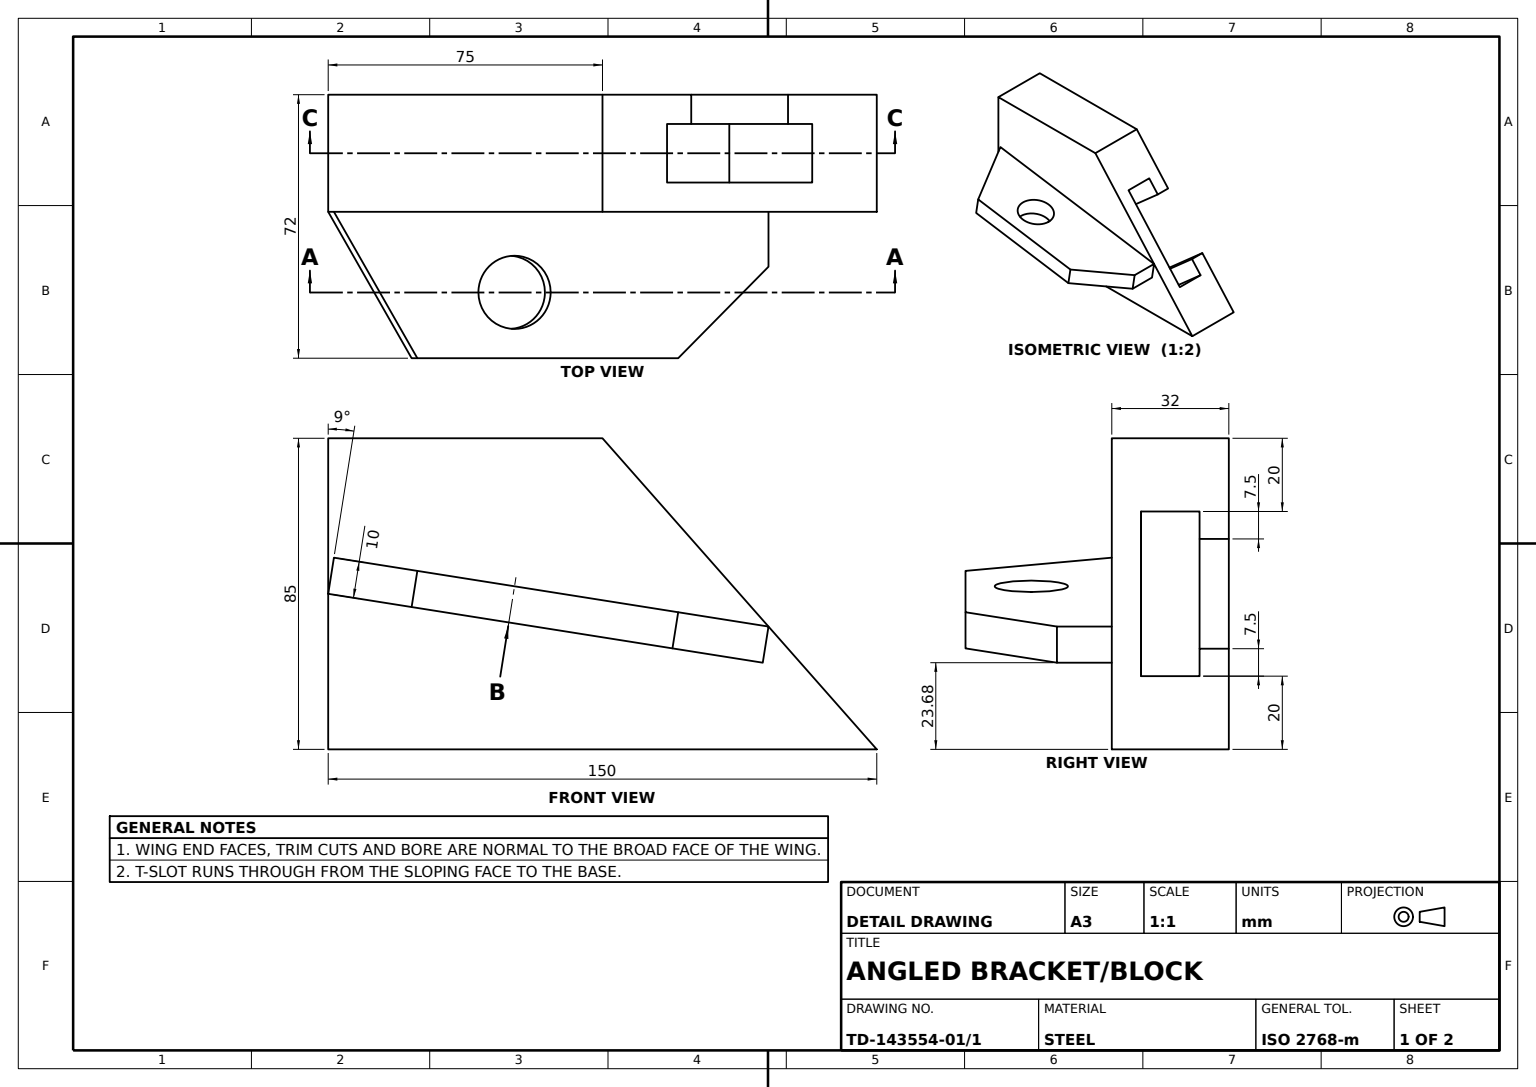
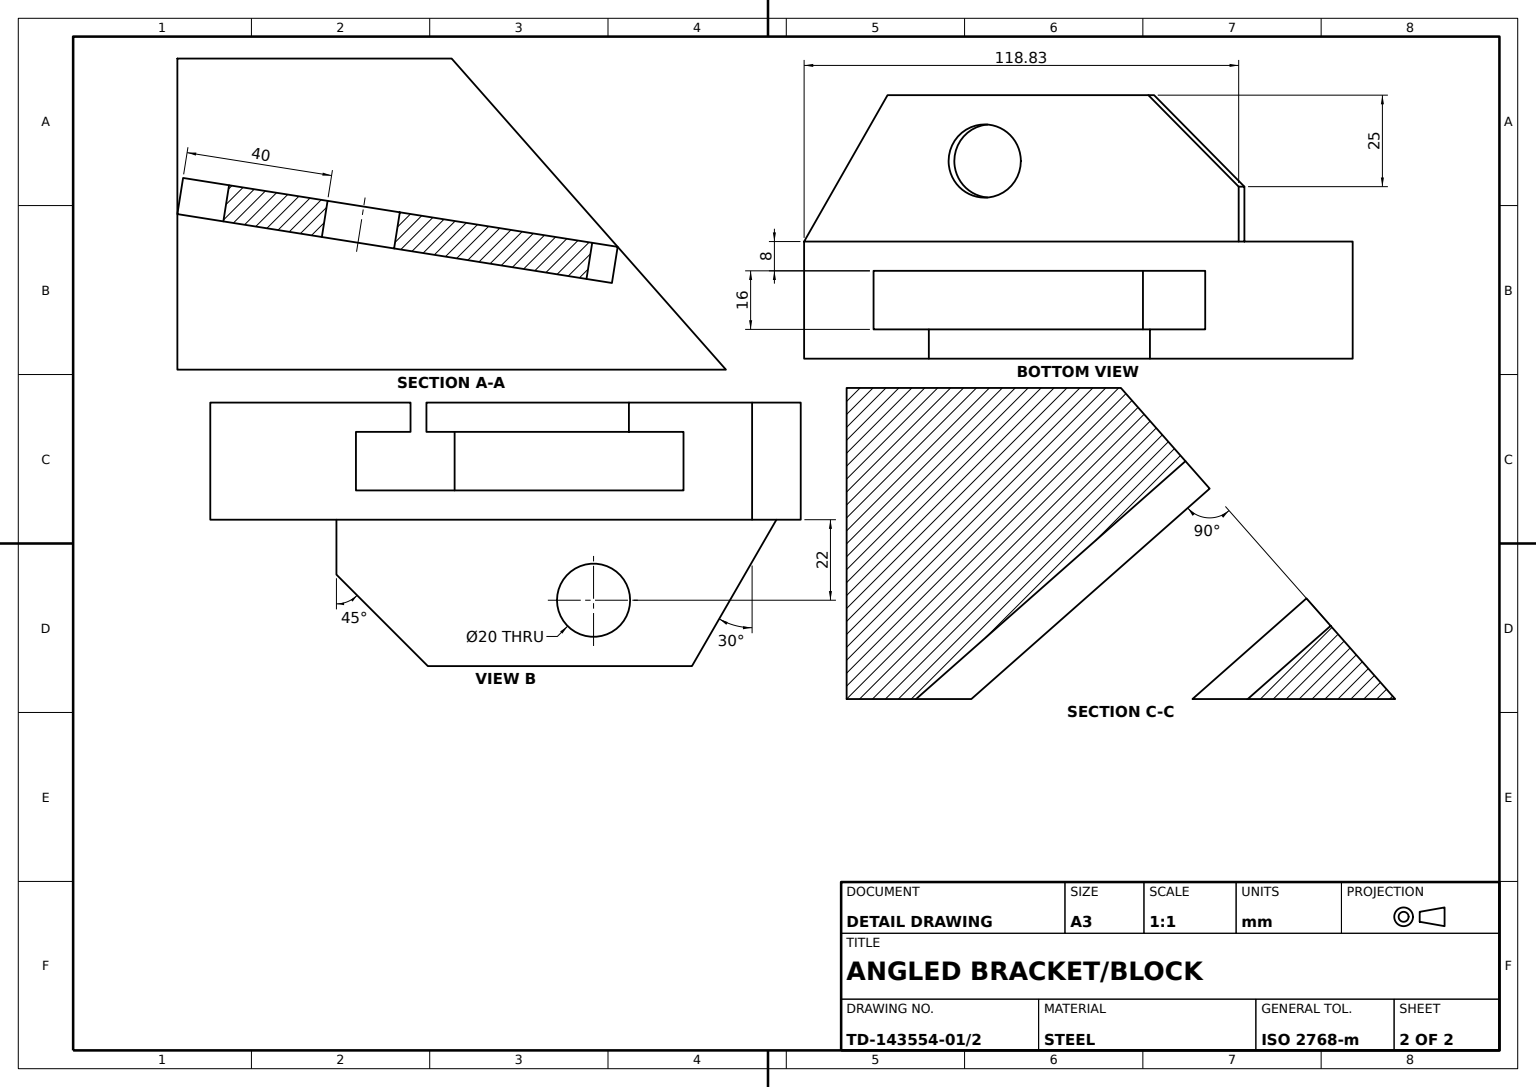
from build123d import *

# Parameters (mm, degrees)
BASE_BLOCK_DEPTH       = 32
SLOT_CUT_DEPTH         = 140
ANGLED_WING_DEPTH      = 40
WING_TRIM_CUT_SKETCH_R = 10
WING_TRIM_CUT_DEPTH    = 40


with BuildPart() as part:
    # Base Block Sketch → Base Block (new body)
    with BuildSketch(Plane.XY):
        Polygon((75, 85), (150, 0), (0, 0), (0, 85), align=None)
    extrude(amount=-BASE_BLOCK_DEPTH)

    # Slot Cut Sketch → Slot Cut (cut)
    with BuildSketch(Plane(origin=(84.338521401, 74.416342412, 0), x_dir=(0, 0, -1), z_dir=(0.7498378553650925, 0.6616216370868463, 0))):
        Polygon((24, -22.564325319), (32, -22.564325319), (32, -62.564325319), (24, -62.564325319), (24, -72.564325319), (8, -72.564325319), (8, -12.564325319), (24, -12.564325319), align=None)
    extrude(amount=-SLOT_CUT_DEPTH, mode=Mode.SUBTRACT)

    # Angled Wing Sketch → Angled Wing (add)
    with BuildSketch(Plane.XY):
        Polygon((120.39128367, 33.556545174), (118.82693902, 23.679661768), (0, 42.5), (1.56434465, 52.376883406), align=None)
    extrude(amount=ANGLED_WING_DEPTH)

    # Wing Trim Cut Sketch → Wing Trim Cut (cut)
    with BuildSketch(Plane(origin=(8.130955781, 51.336834377, 0), x_dir=(0.9876883405951389, -0.15643446504022435, 0), z_dir=(0.15643446504022435, 0.9876883405951389, 0))):
        with Locations(Location((43.351535236, -22, 0), (0, 0, 180))):
            Circle(WING_TRIM_CUT_SKETCH_R)
        Polygon((-6.648464764, 0), (20.17251839, -46.455305531), (-6.648464764, -46.455305531), align=None)
        Polygon((113.659666997, -15), (81.480803865, -47.178863132), (138.076260789, -47.178863132), align=None)
    extrude(amount=-WING_TRIM_CUT_DEPTH, mode=Mode.SUBTRACT)


solid = part.part
